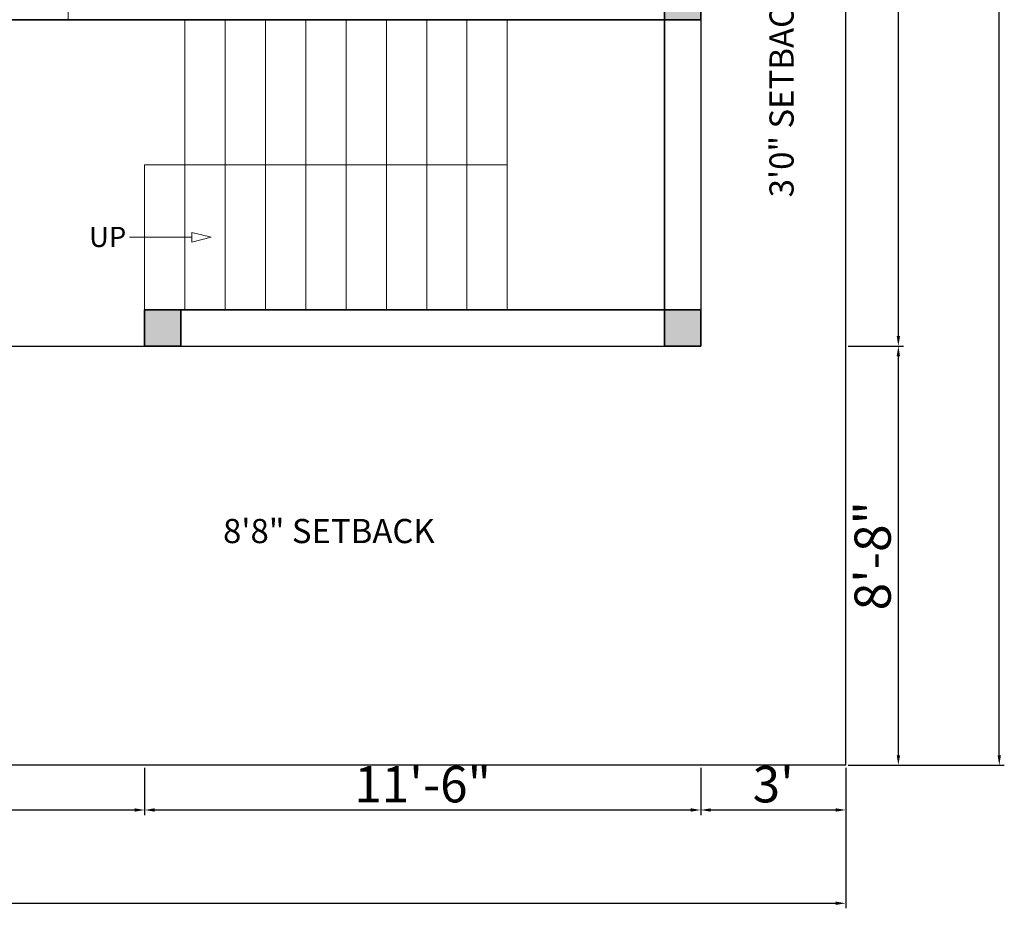
# Model space of a CAD drawing. Units: inches. Extents: x 3321 to 5237, y 11 to 1752.
# Tile 14 of 43: x 4296 to 4541, y 952 to 1172. Entities that reach past the tile are written whole.
import ezdxf

# ---------------------------------------------------------------- set-up
doc = ezdxf.new("R2010")
doc.units = ezdxf.units.IN
for name, color, linetype, lineweight in [('A-ANNO-DIMS', 2, 'Continuous', 18), ('A-ANNO-SYMB', 7, 'Continuous', 18), ('A-ANNO-TEXT', 7, 'Continuous', 18), ('A-COLS', 1, 'Continuous', 35), ('A-FLOR-EDGE', 7, 'Continuous', 25), ('A-FLOR-STRS', 7, 'Continuous', 18), ('A-GLAZ', 5, 'Continuous', 18), ('A-WALL', 7, 'Continuous', 35), ('C-PROP', 7, 'Continuous', 30)]:
    doc.layers.add(name, color=color, linetype=linetype, lineweight=lineweight)
doc.styles.get("Standard").update_dxf_attribs({"font": 'arial.ttf'})
doc.dimstyles.new('ISO-25', dxfattribs={"dimtxt": 9, "dimasz": 2.5, "dimexe": 1.25, "dimexo": 0.625, "dimtad": 1, "dimdec": 1, "dimlunit": 3, "dimtxsty": 'Standard', "dimcen": 2.5, "dimclrd": 4, "dimclre": 4, "dimclrt": 256, "dimadec": 0, "dimazin": 0, "dimtfac": 1, "dimtdec": 1, "dimtmove": 0, "dimatfit": 3, "dimfxl": 1, "dimarcsym": 0})

# ---------------------------------------------------------------- blocks, each defined once
blk = doc.blocks.new('*D57')
at = {"layer": 'A-ANNO-DIMS', "color": 0, "lineweight": -2, "transparency": 16777216}
for p, q in [((4066.39, 986.71), (4066.39, 974.99)), ((4327.39, 986.71), (4327.39, 974.99)), ((4068.89, 976.24), (4324.89, 976.24))]:
    blk.add_line(p, q, dxfattribs=at)
at = {"layer": 'A-ANNO-DIMS', "color": 0, "transparency": 16777216}
for points in [[(4068.89, 976.66), (4068.89, 975.82), (4066.39, 976.24)], [(4324.89, 976.66), (4324.89, 975.82), (4327.39, 976.24)]]:
    blk.add_solid(points, dxfattribs=at)
at = {"layer": 'Defpoints', "color": 0, "transparency": 16777216}
for p in [(4066.39, 987.34), (4327.39, 987.34), (4327.39, 976.24)]:
    blk.add_point(p, dxfattribs=at)
at = {"layer": 'A-ANNO-DIMS', "color": 0, "transparency": 16777216, "insert": (4196.89, 981.46), "char_height": 9, "attachment_point": 5}
blk.add_mtext('21\'-9"', dxfattribs=at)
blk = doc.blocks.new('*D58')
at = {"layer": 'A-ANNO-DIMS', "color": 0, "lineweight": -2, "transparency": 16777216}
for p, q in [((4327.39, 986.71), (4327.39, 974.99)), ((4465.39, 986.71), (4465.39, 974.99)), ((4329.89, 976.24), (4462.89, 976.24))]:
    blk.add_line(p, q, dxfattribs=at)
at = {"layer": 'A-ANNO-DIMS', "color": 0, "transparency": 16777216}
for points in [[(4329.89, 976.66), (4329.89, 975.82), (4327.39, 976.24)], [(4462.89, 976.66), (4462.89, 975.82), (4465.39, 976.24)]]:
    blk.add_solid(points, dxfattribs=at)
at = {"layer": 'Defpoints', "color": 0, "transparency": 16777216}
for p in [(4327.39, 987.34), (4465.39, 987.34), (4465.39, 976.24)]:
    blk.add_point(p, dxfattribs=at)
at = {"layer": 'A-ANNO-DIMS', "color": 0, "transparency": 16777216, "insert": (4396.39, 981.46), "char_height": 9, "attachment_point": 5}
blk.add_mtext('11\'-6"', dxfattribs=at)
blk = doc.blocks.new('*D59')
at = {"layer": 'A-ANNO-DIMS', "color": 0, "lineweight": -2, "transparency": 16777216}
for p, q in [((4465.39, 986.71), (4465.39, 974.99)), ((4501.39, 986.71), (4501.39, 974.99)), ((4467.89, 976.24), (4498.89, 976.24))]:
    blk.add_line(p, q, dxfattribs=at)
at = {"layer": 'A-ANNO-DIMS', "color": 0, "transparency": 16777216}
for points in [[(4467.89, 976.66), (4467.89, 975.82), (4465.39, 976.24)], [(4498.89, 976.66), (4498.89, 975.82), (4501.39, 976.24)]]:
    blk.add_solid(points, dxfattribs=at)
at = {"layer": 'Defpoints', "color": 0, "transparency": 16777216}
for p in [(4465.39, 987.34), (4501.39, 987.34), (4501.39, 976.24)]:
    blk.add_point(p, dxfattribs=at)
at = {"layer": 'A-ANNO-DIMS', "color": 0, "transparency": 16777216, "insert": (4483.39, 981.46), "char_height": 9, "attachment_point": 5}
blk.add_mtext("3'", dxfattribs=at)
blk = doc.blocks.new('*D60')
at = {"layer": 'A-ANNO-DIMS', "color": 0, "lineweight": -2, "transparency": 16777216}
for p, q in [((4502.01, 1091.34), (4515.69, 1091.34)), ((4514.44, 989.84), (4514.44, 1088.84)), ((4502.01, 987.34), (4515.69, 987.34))]:
    blk.add_line(p, q, dxfattribs=at)
at = {"layer": 'A-ANNO-DIMS', "color": 0, "transparency": 16777216}
for points in [[(4514.03, 1088.84), (4514.86, 1088.84), (4514.44, 1091.34)], [(4514.03, 989.84), (4514.86, 989.84), (4514.44, 987.34)]]:
    blk.add_solid(points, dxfattribs=at)
at = {"layer": 'Defpoints', "color": 0, "transparency": 16777216}
for p in [(4501.39, 1091.34), (4514.44, 1091.34), (4501.39, 987.34)]:
    blk.add_point(p, dxfattribs=at)
at = {"layer": 'A-ANNO-DIMS', "color": 0, "transparency": 16777216, "insert": (4509.22, 1039.34), "char_height": 9, "attachment_point": 5, "rotation": 90}
blk.add_mtext('8\'-8"', dxfattribs=at)
blk = doc.blocks.new('*D61')
at = {"layer": 'A-ANNO-DIMS', "color": 0, "lineweight": -2, "transparency": 16777216}
for p, q in [((4502.01, 1687.34), (4515.69, 1687.34)), ((4514.44, 1093.84), (4514.44, 1684.84)), ((4502.01, 1091.34), (4515.69, 1091.34))]:
    blk.add_line(p, q, dxfattribs=at)
at = {"layer": 'A-ANNO-DIMS', "color": 0, "transparency": 16777216}
for points in [[(4514.03, 1684.84), (4514.86, 1684.84), (4514.44, 1687.34)], [(4514.03, 1093.84), (4514.86, 1093.84), (4514.44, 1091.34)]]:
    blk.add_solid(points, dxfattribs=at)
at = {"layer": 'Defpoints', "color": 0, "transparency": 16777216}
for p in [(4501.39, 1687.34), (4514.44, 1687.34), (4501.39, 1091.34)]:
    blk.add_point(p, dxfattribs=at)
at = {"layer": 'A-ANNO-DIMS', "color": 0, "transparency": 16777216, "insert": (4509.22, 1389.34), "char_height": 9, "attachment_point": 5, "rotation": 90}
blk.add_mtext('49\'-8"', dxfattribs=at)
blk = doc.blocks.new('*D64')
at = {"layer": 'A-ANNO-DIMS', "color": 0, "lineweight": -2, "transparency": 16777216}
for p, q in [((4502.01, 1707.34), (4540.73, 1707.34)), ((4539.48, 989.84), (4539.48, 1704.84)), ((4502.01, 987.34), (4540.73, 987.34))]:
    blk.add_line(p, q, dxfattribs=at)
at = {"layer": 'A-ANNO-DIMS', "color": 0, "transparency": 16777216}
for points in [[(4539.06, 1704.84), (4539.9, 1704.84), (4539.48, 1707.34)], [(4539.06, 989.84), (4539.9, 989.84), (4539.48, 987.34)]]:
    blk.add_solid(points, dxfattribs=at)
at = {"layer": 'Defpoints', "color": 0, "transparency": 16777216}
for p in [(4501.39, 1707.34), (4539.48, 1707.34), (4501.39, 987.34)]:
    blk.add_point(p, dxfattribs=at)
at = {"layer": 'A-ANNO-DIMS', "color": 0, "transparency": 16777216, "insert": (4534.26, 1347.34), "char_height": 9, "attachment_point": 5, "rotation": 90}
blk.add_mtext("60'", dxfattribs=at)
blk = doc.blocks.new('*D66')
at = {"layer": 'A-ANNO-DIMS', "color": 0, "lineweight": -2, "transparency": 16777216}
for p, q in [((4021.39, 986.71), (4021.39, 951.84)), ((4501.39, 986.71), (4501.39, 951.84)), ((4023.89, 953.09), (4498.89, 953.09))]:
    blk.add_line(p, q, dxfattribs=at)
at = {"layer": 'A-ANNO-DIMS', "color": 0, "transparency": 16777216}
for points in [[(4023.89, 953.51), (4023.89, 952.68), (4021.39, 953.09)], [(4498.89, 953.51), (4498.89, 952.68), (4501.39, 953.09)]]:
    blk.add_solid(points, dxfattribs=at)
at = {"layer": 'Defpoints', "color": 0, "transparency": 16777216}
for p in [(4021.39, 987.34), (4501.39, 987.34), (4501.39, 953.09)]:
    blk.add_point(p, dxfattribs=at)
at = {"layer": 'A-ANNO-DIMS', "color": 0, "transparency": 16777216, "insert": (4261.39, 958.31), "char_height": 9, "attachment_point": 5}
blk.add_mtext("40'", dxfattribs=at)
blk = doc.blocks.new('COL-9X12-FURN-PLAN')
h = blk.add_hatch(color=256)
h.dxf.hatch_style = 1
h.paths.add_polyline_path([(0, 12), (0, 0), (9, 0), (9, 12)])
blk.add_lwpolyline([(0, 0), (9, 0), (9, 12), (0, 12)], close=True)
blk = doc.blocks.new('COL-9X9-FURN-PLAN')
h = blk.add_hatch(color=256)
h.dxf.hatch_style = 1
h.paths.add_polyline_path([(9, 9), (0, 9), (0, 0), (9, 0)])
blk.add_lwpolyline([(0, 0), (9, 0), (9, 9), (0, 9)], close=True)
blk = doc.blocks.new('WIN-48IN-9IN-WALL')
for p, q in [((0, 0), (0, 9)), ((48, 0), (48, 9)), ((0, 5), (48, 5)), ((0, 4), (48, 4))]:
    blk.add_line(p, q)
blk = doc.blocks.new('STAIR-RETURN-72IN')
for p, q in [((10, 72), (10, 0)), ((20, 72), (20, 0)), ((30, 72), (30, 0)), ((40, 72), (40, 0)), ((50, 72), (50, 0)), ((60, 72), (60, 0)), ((70, 72), (70, 0)), ((80, 72), (80, 0)), ((90, 72), (90, 0)), ((90, 36), (0, 36)), ((0, 36), (0, 0))]:
    blk.add_line(p, q)
blk = doc.blocks.new('STAIR-DIRECTION-ARROW')
blk.add_line((0, 1.22), (15.43, 1.22))
blk.add_lwpolyline([(20.27, 1.22), (15.43, 2.43), (15.43, 0)], close=True)
blk = doc.blocks.new('PROPERTY-40X60FT')
for q in [(480, 720), (0, 0)]:
    blk.add_line((0, 720), q)
blk = doc.blocks.new('*D215')
at = {"layer": 'A-ANNO-DIMS', "color": 4, "lineweight": -2, "transparency": 16777216}
for p, q in [((4221.54, 1180.71), (4221.54, 1173.77)), ((4263.67, 1180.71), (4263.67, 1173.77)), ((4224.04, 1175.02), (4261.17, 1175.02)), ((4263.67, 1175.02), (4342.06, 1175.02))]:
    blk.add_line(p, q, dxfattribs=at)
at = {"layer": 'A-ANNO-DIMS', "color": 4, "transparency": 16777216}
for points in [[(4224.04, 1175.44), (4224.04, 1174.6), (4221.54, 1175.02)], [(4261.17, 1175.44), (4261.17, 1174.6), (4263.67, 1175.02)]]:
    blk.add_solid(points, dxfattribs=at)
at = {"layer": 'Defpoints', "color": 0, "transparency": 16777216}
for p in [(4221.54, 1181.34), (4263.67, 1181.34), (4263.67, 1175.02)]:
    blk.add_point(p, dxfattribs=at)
at = {"layer": 'A-ANNO-DIMS', "transparency": 16777216, "insert": (4304.12, 1180.24), "char_height": 9, "attachment_point": 5}
blk.add_mtext('TV 3\'-6" TYP.', dxfattribs=at)

msp = doc.modelspace()

# ---------------------------------------------------------------- linework, layer by layer
at = {"layer": 'A-FLOR-EDGE'}
for p in [(4465.39, 1687.34), (4066.39, 1091.34)]:
    msp.add_line(p, (4465.39, 1091.34), dxfattribs=at)
at = {"layer": 'A-WALL'}
for p, q in [((4126.39, 1172.34), (4456.39, 1172.34)), ((4456.39, 1172.34), (4456.39, 1100.34)), ((4327.39, 1100.34), (4327.39, 1091.34)), ((4327.39, 1100.34), (4456.39, 1100.34))]:
    msp.add_line(p, q, dxfattribs=at)

# ---------------------------------------------------------------- block references
at = {"layer": 'A-ANNO-SYMB'}
msp.add_blockref('STAIR-DIRECTION-ARROW', (4323.66, 1117.12), dxfattribs=at)
at = {"layer": 'A-COLS'}
for name, p in [('COL-9X12-FURN-PLAN', (4456.39, 1172.34)), ('COL-9X9-FURN-PLAN', (4327.39, 1091.34)), ('COL-9X9-FURN-PLAN', (4456.39, 1091.34))]:
    msp.add_blockref(name, p, dxfattribs=at)
at = {"layer": 'A-FLOR-STRS'}
msp.add_blockref('STAIR-RETURN-72IN', (4327.39, 1100.34), dxfattribs=at)
at = {"layer": 'A-GLAZ'}
msp.add_blockref('WIN-48IN-9IN-WALL', (4260.39, 1172.34), dxfattribs=at)
at = {"layer": 'C-PROP', "rotation": 180}
msp.add_blockref('PROPERTY-40X60FT', (4501.39, 1707.34), dxfattribs=at)

# ---------------------------------------------------------------- texts
at = {"layer": 'A-ANNO-TEXT'}
msp.add_text('UP', height=5, dxfattribs=at).set_placement((4313.6, 1115.94))
at = {"layer": 'A-ANNO-TEXT', "insert": (4482.45, 1128.26), "char_height": 6, "attachment_point": 1, "rotation": 90}
msp.add_mtext_dynamic_manual_height_columns('3\'0" SETBACK', width=97.3114, gutter_width=25, heights=[0], dxfattribs=at)
at = {"layer": 'A-ANNO-TEXT', "insert": (4346.85, 1048.46), "char_height": 6, "attachment_point": 1}
msp.add_mtext_dynamic_manual_height_columns('8\'8" SETBACK', width=97.3114, gutter_width=25, heights=[0], dxfattribs=at)

# ---------------------------------------------------------------- dimensions: what is measured, and where the dimension line sits
at = {"layer": 'A-ANNO-DIMS'}
for base, p1, p2, angle, override, picture, middle in [((4539.48, 1707.34), (4501.39, 987.34), (4501.39, 1707.34), 270, {"dimclrd": 0, "dimclre": 0, "dimclrt": 0}, '*D64', (4534.26, 1347.34)), ((4514.44, 1687.34), (4501.39, 1091.34), (4501.39, 1687.34), 90, {"dimclrd": 0, "dimclre": 0, "dimclrt": 0, "dimtmove": 1}, '*D61', (4509.22, 1389.34)), ((4514.44, 1091.34), (4501.39, 987.34), (4501.39, 1091.34), 90, {"dimclrd": 0, "dimclre": 0, "dimclrt": 0}, '*D60', (4509.22, 1039.34))]:
    dim = msp.add_linear_dim(base=base, p1=p1, p2=p2, angle=angle, dimstyle='ISO-25', override=override, dxfattribs=at)
    dim.commit()
    dim.dimension.update_dxf_attribs({"geometry": picture, "text_midpoint": middle})
dim = msp.add_linear_dim(base=(4263.67, 1175.02), p1=(4221.54, 1181.34), p2=(4263.67, 1181.34), text='TV <> TYP.', dimstyle='ISO-25', override={"dimdec": 1, "dimlfac": 1, "dimrnd": 0, "dimzin": 1, "dimdsep": 46, "dimlunit": 4, "dimfrac": 2}, dxfattribs=at)
dim.commit()
dim.dimension.update_dxf_attribs({"geometry": '*D215', "text_midpoint": (4304.12, 1180.24)})
for base, p1, p2, override, picture, middle in [((4501.39, 953.09), (4021.39, 987.34), (4501.39, 987.34), {"dimclrd": 0, "dimclre": 0, "dimclrt": 0}, '*D66', (4261.39, 958.31)), ((4327.39, 976.24), (4066.39, 987.34), (4327.39, 987.34), {"dimclrd": 0, "dimclre": 0, "dimclrt": 0, "dimtmove": 1}, '*D57', (4196.89, 981.46)), ((4465.39, 976.24), (4327.39, 987.34), (4465.39, 987.34), {"dimclrd": 0, "dimclre": 0, "dimclrt": 0, "dimtmove": 1}, '*D58', (4396.39, 981.46)), ((4501.39, 976.24), (4465.39, 987.34), (4501.39, 987.34), {"dimclrd": 0, "dimclre": 0, "dimclrt": 0, "dimtmove": 1}, '*D59', (4483.39, 981.46))]:
    dim = msp.add_linear_dim(base=base, p1=p1, p2=p2, dimstyle='ISO-25', override=override, dxfattribs=at)
    dim.commit()
    dim.dimension.update_dxf_attribs({"geometry": picture, "text_midpoint": middle})

doc.saveas('drawing.dxf')
